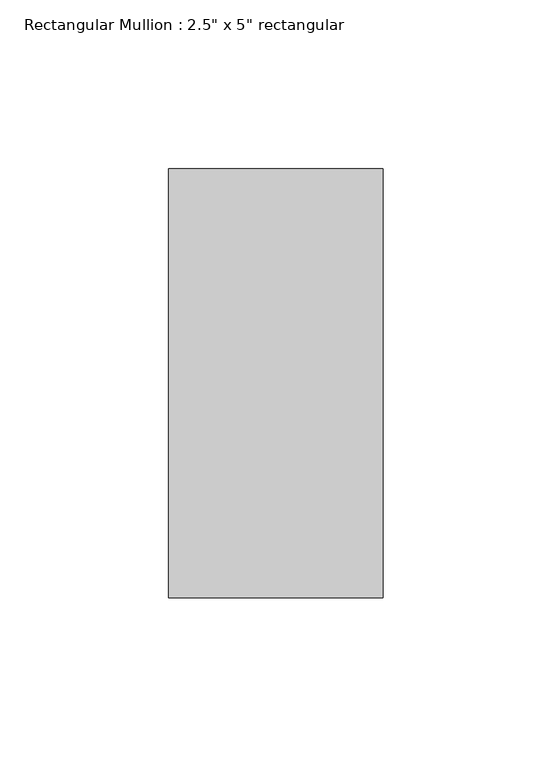
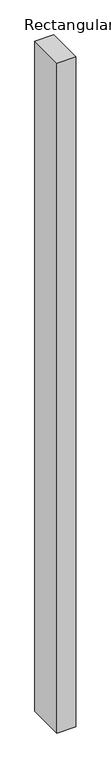
"""IFC4 building model written with IfcOpenShell, lengths in millimetres: member geometry."""

from ifc_helpers import new_model, si_unit, frame, origin, place, context, project, spatial, polyline, outline, extrude, source, transform, mapped, element, save


def member_6a1115f2(model_context):
    return source(origin(), model_context, "Body", "SweptSolid", [
        extrude(outline(polyline([(0.0, 63.5), (0.0, -63.5), (-63.5, -63.5), (-63.5, 63.5), (0.0, 63.5)])), frame((0.0, 0.0, -2364.5663272), z_axis=(0.0, 0.0, 1.0), x_axis=(1.0, 0.0, 0.0)), (0.0, 0.0, 1.0), 2364.5663272),
    ])


if __name__ == "__main__":
    model = new_model("IFC4")
    model_context = context("Model", 3, world=origin())
    ifc_project = project(units=[si_unit("LENGTHUNIT", "METRE", prefix="MILLI")], contexts=[model_context])
    site = spatial("IfcSite", under=ifc_project)
    building = spatial("IfcBuilding", under=site)
    placement = place(None, origin())
    member_shape = member_6a1115f2(model_context)
    element("IfcMember", 1, ObjectType="Rectangular Mullion : 2.5\" x 5\" rectangular", at=placement, inside=building, context=model_context, shape_type="MappedRepresentation", body=[
        mapped(member_shape, transform((0.0, 0.0, 0.0), x_axis=(1.0, 0.0, 0.0), y_axis=(0.0, 1.0, 0.0), z_axis=(0.0, 0.0, 1.0))),
    ])
    save(model, "model.ifc")

# Revit data of these elements
# Type "Rectangular Mullion : 2.5\" x 5\" rectangular"
#   built-in parameter 1007304 = 0.416667 (stored number, unit not read)
#   built-in parameter 1007301 = 0.104167 (stored number, unit not read)
#   built-in parameter 1007300 = 0.104167 (stored number, unit not read)
# Element 1 (IfcMember, "Rectangular Mullion : 2.5\" x 5\" rectangular")
#   Materials on its faces: "Aluminum"
# Materials
#   "Aluminum": class "Metal", colour RGB 247 247 247, transparency 0, Description = "Aluminum 6061", Cost = 0
